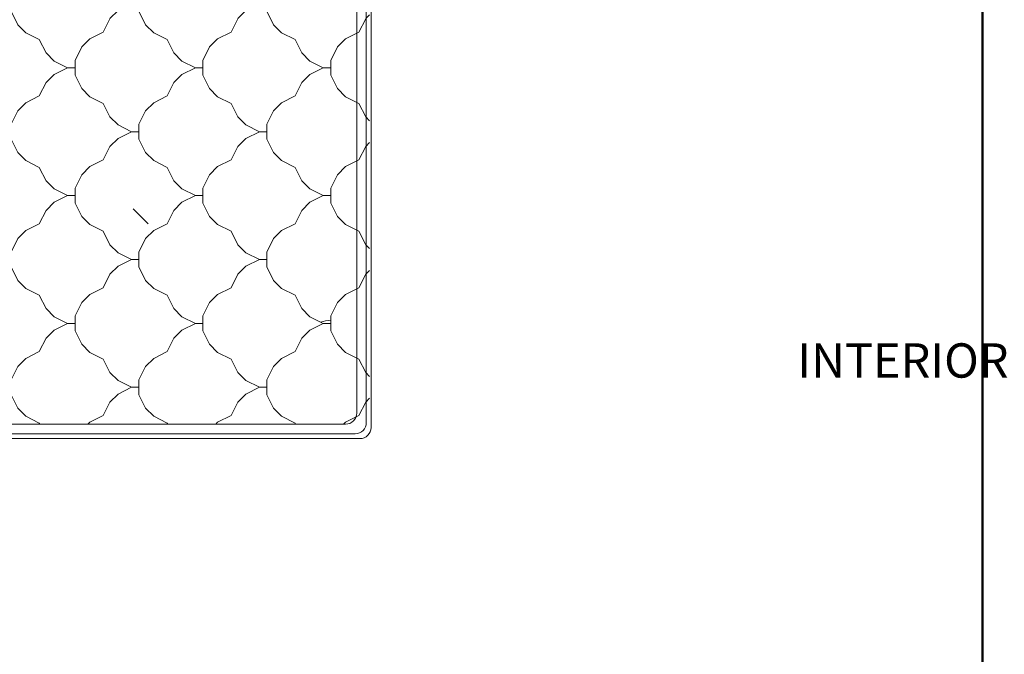
# Model space of a CAD drawing. Units: inches. Extents: x 513 to 1142, y 396 to 927.
# Tile 8 of 31: x 628 to 743, y 746 to 820. Entities that reach past the tile are written whole.
import ezdxf

# ---------------------------------------------------------------- set-up
doc = ezdxf.new("R2010")
doc.units = ezdxf.units.IN
doc.header["$MEASUREMENT"] = 0
doc.linetypes.add('DASHED', pattern=[0.75, 0.5, -0.25])
for name, color, linetype, lineweight in [('A-ANNO-DIMS', 2, 'DASHED', 18), ('A-WALL', 7, 'Continuous', 50), ('furniture', 92, 'Continuous', 18)]:
    doc.layers.add(name, color=color, linetype=linetype, lineweight=lineweight)
doc.styles.get("Standard").update_dxf_attribs({"font": 'arial.ttf'})
doc.dimstyles.get("Standard").update_dxf_attribs({"dimtxt": 4, "dimasz": 0.18, "dimexe": 0.18, "dimexo": 0.0625, "dimgap": 0.09, "dimtad": 0, "dimtih": 1, "dimtoh": 1, "dimdec": 0, "dimrnd": 6, "dimzin": 0, "dimdsep": 46, "dimlunit": 3, "dimtxsty": 'Standard', "dimcen": 0.09, "dimadec": 0, "dimazin": 0, "dimtfac": 1, "dimtdec": 0, "dimtofl": 0, "dimtmove": 0, "dimatfit": 3, "dimfxl": 1, "dimtolj": 1, "dimtzin": 0, "dimarcsym": 0})

# ---------------------------------------------------------------- blocks, each defined once
blk = doc.blocks.new('A$C029D5C69')
for p, q in [((0.4164, 2.0693), (0.4164, 2.0066)), ((2.2315, 2.0693), (0.4164, 2.0693)), ((2.2315, 2.0066), (2.2315, 2.0693)), ((0, 1.606), (0, 2.0066)), ((0, 2.0066), (0.505, 2.0066)), ((0.0151, 1.6211), (0.0151, 1.9915)), ((0.0151, 1.9915), (0.4899, 1.9915)), ((0.4164, 2.0066), (2.2315, 2.0066)), ((0.4899, 1.9915), (0.4899, 1.6211)), ((0.505, 2.0066), (0.505, 1.606)), ((0.5252, 0.0351), (0.5252, 2.0066)), ((0.5403, 0.0502), (0.5403, 2.0066)), ((0.5706, 0.0805), (0.5706, 2.0066)), ((0.6869, 1.966), (0.6666, 2.0066)), ((0.7072, 2.0066), (0.6869, 1.966)), ((1.0902, 1.966), (1.0699, 2.0066)), ((1.1106, 2.0066), (1.0902, 1.966)), ((2.1114, 2.0087), (2.1114, 0.0351)), ((2.6479, 2.0066), (2.1429, 2.0066)), ((2.1429, 2.0066), (2.1429, 1.606)), ((2.6328, 1.9915), (2.158, 1.9915)), ((2.158, 1.9915), (2.158, 1.6211)), ((2.6328, 1.6211), (2.6328, 1.9915)), ((2.6479, 1.606), (2.6479, 2.0066)), ((0.2689, 1.9609), (0.2689, 1.6764)), ((0.6869, 1.9425), (0.6869, 1.966)), ((0.6869, 1.9425), (0.6869, 1.966)), ((1.0902, 1.9425), (1.0902, 1.966)), ((1.0902, 1.9425), (1.0902, 1.966)), ((1.8954, 1.9865), (1.3081, 1.9865)), ((1.8954, 1.9713), (1.3339, 1.9713)), ((1.3849, 1.9713), (1.3656, 1.952)), ((1.3945, 1.9713), (1.3714, 1.9483)), ((1.4249, 1.945), (1.3986, 1.9713)), ((1.4288, 1.9507), (1.4081, 1.9713)), ((1.487, 1.9713), (1.4664, 1.9507)), ((1.4966, 1.9713), (1.4703, 1.945)), ((1.527, 1.945), (1.5007, 1.9713)), ((1.5309, 1.9507), (1.5102, 1.9713)), ((1.5891, 1.9713), (1.5685, 1.9507)), ((1.5987, 1.9713), (1.5724, 1.945)), ((1.6291, 1.945), (1.6028, 1.9713)), ((1.633, 1.9507), (1.6123, 1.9713)), ((1.6912, 1.9713), (1.6706, 1.9507)), ((1.7008, 1.9713), (1.6745, 1.945)), ((1.7312, 1.945), (1.7049, 1.9713)), ((1.7351, 1.9507), (1.7144, 1.9713)), ((1.7933, 1.9713), (1.7727, 1.9507)), ((1.8029, 1.9713), (1.7766, 1.945)), ((1.8333, 1.945), (1.807, 1.9713)), ((1.8372, 1.9507), (1.8165, 1.9713)), ((1.8954, 1.9713), (1.8748, 1.9507)), ((1.9043, 1.9707), (1.8787, 1.945)), ((1.9354, 1.945), (1.9114, 1.969)), ((2.379, 1.9609), (2.379, 1.6764)), ((0.6634, 1.9425), (0.621, 1.9213)), ((0.6634, 1.9425), (0.621, 1.9213)), ((0.6869, 1.9425), (0.6634, 1.9425)), ((0.6869, 1.9425), (0.7104, 1.9425)), ((0.7528, 1.9213), (0.7104, 1.9425)), ((0.7528, 1.9213), (0.7104, 1.9425)), ((1.0668, 1.9425), (1.0244, 1.9213)), ((1.0668, 1.9425), (1.0244, 1.9213)), ((1.0902, 1.9425), (1.0668, 1.9425)), ((1.0902, 1.9425), (1.1137, 1.9425)), ((1.1561, 1.9213), (1.1137, 1.9425)), ((1.1561, 1.9213), (1.1137, 1.9425)), ((1.4249, 1.945), (1.4059, 1.926)), ((1.4288, 1.9394), (1.4116, 1.9222)), ((1.4476, 1.9507), (1.4288, 1.9507)), ((1.4288, 1.9393), (1.4476, 1.9393)), ((1.4476, 1.9507), (1.4664, 1.9507)), ((1.4664, 1.9393), (1.4476, 1.9393)), ((1.493, 1.9128), (1.4664, 1.9394)), ((1.4986, 1.9167), (1.4703, 1.945)), ((1.527, 1.945), (1.4986, 1.9167)), ((1.5309, 1.9394), (1.5043, 1.9128)), ((1.5497, 1.9507), (1.5309, 1.9507)), ((1.5309, 1.9393), (1.5497, 1.9393)), ((1.5497, 1.9507), (1.5685, 1.9507)), ((1.5685, 1.9393), (1.5497, 1.9393)), ((1.595, 1.9128), (1.5685, 1.9394)), ((1.6007, 1.9167), (1.5724, 1.945)), ((1.6291, 1.945), (1.6007, 1.9167)), ((1.633, 1.9394), (1.6064, 1.9128)), ((1.6518, 1.9507), (1.633, 1.9507)), ((1.633, 1.9393), (1.6518, 1.9393)), ((1.6518, 1.9507), (1.6706, 1.9507)), ((1.6706, 1.9393), (1.6518, 1.9393)), ((1.6971, 1.9128), (1.6706, 1.9394)), ((1.7028, 1.9167), (1.6745, 1.945)), ((1.7312, 1.945), (1.7028, 1.9167)), ((1.7351, 1.9394), (1.7085, 1.9128)), ((1.7539, 1.9507), (1.7351, 1.9507)), ((1.7351, 1.9393), (1.7539, 1.9393)), ((1.7539, 1.9507), (1.7727, 1.9507)), ((1.7727, 1.9393), (1.7539, 1.9393)), ((1.7992, 1.9128), (1.7727, 1.9394)), ((1.8049, 1.9167), (1.7766, 1.945)), ((1.8333, 1.945), (1.8049, 1.9167)), ((1.8372, 1.9394), (1.8106, 1.9128)), ((1.856, 1.9507), (1.8372, 1.9507)), ((1.8372, 1.9393), (1.856, 1.9393)), ((1.856, 1.9507), (1.8748, 1.9507)), ((1.8748, 1.9393), (1.856, 1.9393)), ((1.9013, 1.9128), (1.8748, 1.9394)), ((1.907, 1.9167), (1.8787, 1.945)), ((1.9354, 1.945), (1.907, 1.9167)), ((1.9393, 1.9394), (1.9127, 1.9128)), ((1.9393, 1.9393), (1.9404, 1.9393)), ((1.9414, 1.688), (1.9414, 1.931)), ((1.9565, 1.688), (1.9565, 1.931)), ((0.5955, 1.8958), (0.5743, 1.8534)), ((0.621, 1.9213), (0.5955, 1.8958)), ((0.7783, 1.8958), (0.7528, 1.9213)), ((0.7995, 1.8534), (0.7783, 1.8958)), ((0.9989, 1.8958), (0.9777, 1.8534)), ((1.0243, 1.9213), (0.9988, 1.8958)), ((1.1816, 1.8958), (1.1561, 1.9213)), ((1.2028, 1.8534), (1.1816, 1.8958)), ((1.493, 1.8752), (1.493, 1.9128)), ((1.5043, 1.8752), (1.5043, 1.9128)), ((1.595, 1.8752), (1.595, 1.9128)), ((1.6064, 1.8752), (1.6064, 1.9128)), ((1.6971, 1.8752), (1.6971, 1.9128)), ((1.7085, 1.8752), (1.7085, 1.9128)), ((1.7992, 1.8752), (1.7992, 1.9128)), ((1.8106, 1.8752), (1.8106, 1.9128)), ((1.9013, 1.8752), (1.9013, 1.9128)), ((1.9127, 1.8752), (1.9127, 1.9128)), ((1.493, 1.8752), (1.4867, 1.869)), ((1.4986, 1.8713), (1.4922, 1.8648)), ((1.527, 1.8429), (1.4986, 1.8713)), ((1.5309, 1.8486), (1.5043, 1.8752)), ((1.595, 1.8752), (1.5685, 1.8486)), ((1.6007, 1.8713), (1.5724, 1.8429)), ((1.6291, 1.8429), (1.6007, 1.8713)), ((1.633, 1.8486), (1.6064, 1.8752)), ((1.6971, 1.8752), (1.6706, 1.8486)), ((1.7028, 1.8713), (1.6745, 1.8429)), ((1.7312, 1.8429), (1.7028, 1.8713)), ((1.7351, 1.8486), (1.7085, 1.8752)), ((1.7992, 1.8752), (1.7727, 1.8486)), ((1.8049, 1.8713), (1.7766, 1.8429)), ((1.8333, 1.8429), (1.8049, 1.8713)), ((1.8372, 1.8486), (1.8106, 1.8752)), ((1.9013, 1.8752), (1.8748, 1.8486)), ((1.907, 1.8713), (1.8787, 1.8429)), ((1.9354, 1.8429), (1.907, 1.8713)), ((1.9393, 1.8486), (1.9127, 1.8752)), ((0.5743, 1.8534), (0.5706, 1.8515)), ((0.5743, 1.8534), (0.5706, 1.8515)), ((0.8419, 1.8322), (0.7995, 1.8534)), ((0.8419, 1.8322), (0.7995, 1.8534)), ((0.9777, 1.8534), (0.9353, 1.8322)), ((0.9777, 1.8534), (0.9353, 1.8322)), ((1.2452, 1.8322), (1.2028, 1.8534)), ((1.2452, 1.8322), (1.2028, 1.8534)), ((1.527, 1.8429), (1.5242, 1.8401)), ((1.5309, 1.8373), (1.5295, 1.8359)), ((1.5497, 1.8486), (1.5309, 1.8486)), ((1.5309, 1.8373), (1.5497, 1.8373)), ((1.5497, 1.8486), (1.5685, 1.8486)), ((1.5685, 1.8373), (1.5497, 1.8373)), ((1.595, 1.8107), (1.5685, 1.8373)), ((1.6007, 1.8146), (1.5724, 1.8429)), ((1.6291, 1.8429), (1.6007, 1.8146)), ((1.633, 1.8373), (1.6064, 1.8107)), ((1.6518, 1.8486), (1.633, 1.8486)), ((1.633, 1.8373), (1.6518, 1.8373)), ((1.6518, 1.8486), (1.6706, 1.8486)), ((1.6706, 1.8373), (1.6518, 1.8373)), ((1.6971, 1.8107), (1.6706, 1.8373)), ((1.7028, 1.8146), (1.6745, 1.8429)), ((1.7312, 1.8429), (1.7028, 1.8146)), ((1.7351, 1.8373), (1.7085, 1.8107)), ((1.7539, 1.8486), (1.7351, 1.8486)), ((1.7351, 1.8373), (1.7539, 1.8373)), ((1.7539, 1.8486), (1.7727, 1.8486)), ((1.7727, 1.8373), (1.7539, 1.8373)), ((1.7992, 1.8107), (1.7727, 1.8373)), ((1.8049, 1.8146), (1.7766, 1.8429)), ((1.8333, 1.8429), (1.8049, 1.8146)), ((1.8372, 1.8373), (1.8106, 1.8107)), ((1.856, 1.8486), (1.8372, 1.8486)), ((1.8372, 1.8373), (1.856, 1.8373)), ((1.856, 1.8486), (1.8748, 1.8486)), ((1.8748, 1.8373), (1.856, 1.8373)), ((1.9013, 1.8107), (1.8748, 1.8373)), ((1.907, 1.8146), (1.8787, 1.8429)), ((1.9354, 1.8429), (1.907, 1.8146)), ((1.9393, 1.8373), (1.9127, 1.8107)), ((1.9414, 1.8486), (1.9393, 1.8486)), ((1.9393, 1.8373), (1.9414, 1.8373)), ((0.1267, 1.8186), (0.4111, 1.8186)), ((0.8674, 1.8067), (0.8419, 1.8322)), ((0.8886, 1.7643), (0.8674, 1.8067)), ((0.9098, 1.8067), (0.8886, 1.7643)), ((0.9352, 1.8322), (0.9097, 1.8067)), ((1.2707, 1.8067), (1.2452, 1.8322)), ((1.2919, 1.7643), (1.2707, 1.8067)), ((1.595, 1.7806), (1.595, 1.8107)), ((1.6064, 1.7731), (1.6064, 1.8107)), ((1.6971, 1.7731), (1.6971, 1.8107)), ((1.7085, 1.7731), (1.7085, 1.8107)), ((1.7992, 1.7731), (1.7992, 1.8107)), ((1.8106, 1.7731), (1.8106, 1.8107)), ((1.9013, 1.7731), (1.9013, 1.8107)), ((1.9127, 1.7731), (1.9127, 1.8107)), ((2.2367, 1.8186), (2.5212, 1.8186)), ((1.2981, 1.7768), (1.2919, 1.7643)), ((1.633, 1.7465), (1.6064, 1.7731)), ((1.6971, 1.7731), (1.6706, 1.7465)), ((1.7351, 1.7465), (1.7085, 1.7731)), ((1.7992, 1.7731), (1.7727, 1.7465)), ((1.8372, 1.7465), (1.8106, 1.7731)), ((1.9013, 1.7731), (1.8748, 1.7465)), ((1.9393, 1.7465), (1.9127, 1.7731)), ((0.8651, 1.7408), (0.8227, 1.7196)), ((0.8651, 1.7408), (0.8227, 1.7196)), ((0.912, 1.7408), (0.8651, 1.7408)), ((0.8886, 1.7408), (0.8886, 1.7643)), ((0.9544, 1.7196), (0.912, 1.7408)), ((0.9544, 1.7196), (0.912, 1.7408)), ((1.2684, 1.7408), (1.226, 1.7196)), ((1.2684, 1.7408), (1.226, 1.7196)), ((1.2885, 1.7408), (1.2684, 1.7408)), ((1.2919, 1.7519), (1.2919, 1.7643)), ((1.6518, 1.7465), (1.633, 1.7465)), ((1.6518, 1.7465), (1.6706, 1.7465)), ((1.7028, 1.7692), (1.6745, 1.7408)), ((1.7028, 1.7125), (1.6745, 1.7408)), ((1.7312, 1.7408), (1.7028, 1.7692)), ((1.7312, 1.7408), (1.7028, 1.7125)), ((1.7539, 1.7465), (1.7351, 1.7465)), ((1.7539, 1.7465), (1.7727, 1.7465)), ((1.8049, 1.7692), (1.7766, 1.7408)), ((1.8049, 1.7125), (1.7766, 1.7408)), ((1.8333, 1.7408), (1.8049, 1.7692)), ((1.8333, 1.7408), (1.8049, 1.7125)), ((1.856, 1.7465), (1.8372, 1.7465)), ((1.856, 1.7465), (1.8748, 1.7465)), ((1.907, 1.7692), (1.8787, 1.7408)), ((1.907, 1.7125), (1.8787, 1.7408)), ((1.9354, 1.7408), (1.907, 1.7692)), ((1.9354, 1.7408), (1.907, 1.7125)), ((1.9414, 1.7465), (1.9393, 1.7465)), ((0.8227, 1.7196), (0.7972, 1.6941)), ((0.98, 1.6941), (0.9545, 1.7196)), ((1.226, 1.7196), (1.2005, 1.6941)), ((1.6443, 1.7352), (1.6518, 1.7352)), ((1.6706, 1.7352), (1.6518, 1.7352)), ((1.6971, 1.7086), (1.6706, 1.7352)), ((1.6971, 1.682), (1.6971, 1.7086)), ((1.7351, 1.7352), (1.7085, 1.7086)), ((1.7085, 1.671), (1.7085, 1.7086)), ((1.7351, 1.7352), (1.7539, 1.7352)), ((1.7727, 1.7352), (1.7539, 1.7352)), ((1.7992, 1.7086), (1.7727, 1.7352)), ((1.7992, 1.671), (1.7992, 1.7086)), ((1.8372, 1.7352), (1.8106, 1.7086)), ((1.8106, 1.671), (1.8106, 1.7086)), ((1.8372, 1.7352), (1.856, 1.7352)), ((1.8748, 1.7352), (1.856, 1.7352)), ((1.9013, 1.7086), (1.8748, 1.7352)), ((1.9013, 1.671), (1.9013, 1.7086)), ((1.9393, 1.7352), (1.9127, 1.7086)), ((1.9127, 1.671), (1.9127, 1.7086)), ((1.9393, 1.7352), (1.9414, 1.7352)), ((0.5766, 1.6941), (0.5706, 1.7002)), ((0.5978, 1.6517), (0.5766, 1.6941)), ((0.7972, 1.6941), (0.776, 1.6517)), ((1.0011, 1.6517), (0.9799, 1.6941)), ((1.2005, 1.6941), (1.1793, 1.6517)), ((2.5551, 1.6275), (2.5551, 1.696)), ((0.6402, 1.6305), (0.5978, 1.6517)), ((0.6402, 1.6305), (0.5978, 1.6517)), ((0.776, 1.6517), (0.7336, 1.6305)), ((0.776, 1.6517), (0.7336, 1.6305)), ((1.0435, 1.6305), (1.0011, 1.6517)), ((1.0435, 1.6305), (1.0011, 1.6517)), ((1.1793, 1.6517), (1.1369, 1.6305)), ((1.1793, 1.6517), (1.1369, 1.6305)), ((1.7318, 1.6477), (1.7085, 1.671)), ((1.8961, 1.6477), (1.7289, 1.6477)), ((1.7992, 1.671), (1.7759, 1.6477)), ((1.8049, 1.6671), (1.7855, 1.6477)), ((1.8244, 1.6477), (1.8049, 1.6671)), ((1.8339, 1.6477), (1.8106, 1.671)), ((1.9013, 1.671), (1.878, 1.6477)), ((1.907, 1.6671), (1.8876, 1.6477)), ((1.9202, 1.6539), (1.907, 1.6671)), ((1.926, 1.6577), (1.9127, 1.671)), ((0.4899, 1.6211), (0.0151, 1.6211)), ((0.6657, 1.605), (0.6402, 1.6305)), ((0.7336, 1.6305), (0.7081, 1.605)), ((1.0691, 1.605), (1.0436, 1.6305)), ((1.1369, 1.6305), (1.1114, 1.605)), ((1.8961, 1.6325), (1.7422, 1.6325)), ((2.158, 1.6211), (2.6328, 1.6211)), ((0.505, 1.606), (0, 1.606)), ((0.6869, 1.5626), (0.6657, 1.605)), ((0.7081, 1.605), (0.6869, 1.5626)), ((1.0902, 1.5626), (1.069, 1.605)), ((1.1114, 1.605), (1.0902, 1.5626)), ((2.1429, 1.606), (2.6479, 1.606)), ((0.6869, 1.5392), (0.6869, 1.5626)), ((0.6869, 1.5392), (0.6869, 1.5626)), ((1.0902, 1.5392), (1.0902, 1.5626)), ((1.0902, 1.5392), (1.0902, 1.5626)), ((0.6634, 1.5391), (0.621, 1.5179)), ((0.6634, 1.5391), (0.621, 1.5179)), ((0.6869, 1.5392), (0.6634, 1.5392)), ((0.6869, 1.5392), (0.7104, 1.5392)), ((0.7528, 1.5179), (0.7104, 1.5391)), ((0.7528, 1.5179), (0.7104, 1.5391)), ((1.0668, 1.5391), (1.0244, 1.5179)), ((1.0668, 1.5391), (1.0244, 1.5179)), ((1.0902, 1.5392), (1.0668, 1.5392)), ((1.0902, 1.5392), (1.1137, 1.5392)), ((1.1561, 1.5179), (1.1137, 1.5391)), ((1.1561, 1.5179), (1.1137, 1.5391)), ((1.4534, 1.5308), (1.4277, 1.5179)), ((1.4534, 1.5308), (1.4277, 1.5179)), ((0.5955, 1.4925), (0.5743, 1.4501)), ((0.621, 1.5179), (0.5955, 1.4924)), ((0.7783, 1.4924), (0.7528, 1.5179)), ((0.7995, 1.4501), (0.7783, 1.4925)), ((0.9989, 1.4925), (0.9777, 1.4501)), ((1.0243, 1.5179), (0.9988, 1.4924)), ((1.1816, 1.4924), (1.1561, 1.5179)), ((1.2028, 1.4501), (1.1816, 1.4925)), ((1.4022, 1.4925), (1.381, 1.4501)), ((1.4277, 1.5179), (1.4022, 1.4924)), ((1.6062, 1.4501), (1.5966, 1.4692)), ((0.5743, 1.45), (0.5706, 1.4481)), ((0.5743, 1.45), (0.5706, 1.4481)), ((0.8419, 1.4288), (0.7995, 1.45)), ((0.8419, 1.4288), (0.7995, 1.45)), ((0.8674, 1.4033), (0.8419, 1.4288)), ((0.9352, 1.4288), (0.9097, 1.4033)), ((0.9777, 1.45), (0.9353, 1.4288)), ((0.9777, 1.45), (0.9353, 1.4288)), ((1.2452, 1.4288), (1.2028, 1.45)), ((1.2452, 1.4288), (1.2028, 1.45)), ((1.2707, 1.4033), (1.2452, 1.4288)), ((1.3386, 1.4288), (1.3131, 1.4033)), ((1.381, 1.45), (1.3386, 1.4288)), ((1.381, 1.45), (1.3386, 1.4288)), ((1.6486, 1.4288), (1.6062, 1.45)), ((1.6486, 1.4288), (1.6062, 1.45)), ((1.6741, 1.4033), (1.6486, 1.4288)), ((0.5403, 1.4117), (0.5706, 1.4117)), ((0.8886, 1.361), (0.8674, 1.4034)), ((0.9098, 1.4034), (0.8886, 1.361)), ((1.2919, 1.361), (1.2707, 1.4034)), ((1.3131, 1.4034), (1.2919, 1.361)), ((1.6953, 1.361), (1.6741, 1.4034)), ((1.714, 1.3984), (1.6953, 1.361)), ((0.8651, 1.3374), (0.8227, 1.3162)), ((0.8651, 1.3374), (0.8227, 1.3162)), ((0.912, 1.3375), (0.8651, 1.3375)), ((0.8886, 1.3375), (0.8886, 1.3609)), ((0.9544, 1.3162), (0.912, 1.3374)), ((0.9544, 1.3162), (0.912, 1.3374)), ((1.2684, 1.3374), (1.226, 1.3162)), ((1.2684, 1.3374), (1.226, 1.3162)), ((1.3154, 1.3375), (1.2684, 1.3375)), ((1.2919, 1.3375), (1.2919, 1.3609)), ((1.3578, 1.3162), (1.3154, 1.3374)), ((1.3578, 1.3162), (1.3154, 1.3374)), ((1.6718, 1.3374), (1.6294, 1.3162)), ((1.6718, 1.3374), (1.6294, 1.3162)), ((1.7187, 1.3375), (1.6718, 1.3375)), ((1.6953, 1.3375), (1.6953, 1.3609)), ((1.7611, 1.3162), (1.7187, 1.3374)), ((1.7611, 1.3162), (1.7187, 1.3374)), ((0.8227, 1.3163), (0.7972, 1.2908)), ((0.98, 1.2908), (0.9545, 1.3163)), ((1.226, 1.3163), (1.2005, 1.2908)), ((1.3833, 1.2908), (1.3578, 1.3163)), ((1.6294, 1.3163), (1.6039, 1.2908)), ((1.7867, 1.2908), (1.7611, 1.3163)), ((0.5766, 1.2908), (0.5706, 1.2968)), ((0.5978, 1.2484), (0.5766, 1.2908)), ((0.7972, 1.2908), (0.776, 1.2484)), ((1.0011, 1.2484), (0.9799, 1.2908)), ((1.2005, 1.2908), (1.1793, 1.2484)), ((1.4045, 1.2484), (1.3833, 1.2908)), ((1.6039, 1.2908), (1.5827, 1.2484)), ((1.8078, 1.2484), (1.7866, 1.2908)), ((0.6402, 1.2271), (0.5978, 1.2483)), ((0.6402, 1.2271), (0.5978, 1.2483)), ((0.776, 1.2483), (0.7336, 1.2271)), ((0.776, 1.2483), (0.7336, 1.2271)), ((1.0435, 1.2271), (1.0011, 1.2483)), ((1.0435, 1.2271), (1.0011, 1.2483)), ((1.1793, 1.2483), (1.1369, 1.2271)), ((1.1793, 1.2483), (1.1369, 1.2271)), ((1.4469, 1.2271), (1.4045, 1.2483)), ((1.4469, 1.2271), (1.4045, 1.2483)), ((1.5827, 1.2483), (1.5403, 1.2271)), ((1.5827, 1.2483), (1.5403, 1.2271)), ((1.8502, 1.2271), (1.8078, 1.2483)), ((1.8502, 1.2271), (1.8078, 1.2483)), ((0.6657, 1.2017), (0.6402, 1.2272)), ((0.7336, 1.2272), (0.7081, 1.2017)), ((1.0691, 1.2017), (1.0436, 1.2272)), ((1.1369, 1.2272), (1.1114, 1.2017)), ((1.4724, 1.2017), (1.4469, 1.2272)), ((1.5403, 1.2272), (1.5148, 1.2017)), ((1.8758, 1.2017), (1.8503, 1.2272)), ((0.5403, 1.21), (0.5706, 1.21)), ((0.6869, 1.1593), (0.6657, 1.2017)), ((0.7081, 1.2017), (0.6869, 1.1593)), ((1.0902, 1.1593), (1.069, 1.2017)), ((1.1114, 1.2017), (1.0902, 1.1593)), ((1.4936, 1.1593), (1.4724, 1.2017)), ((1.5148, 1.2017), (1.4936, 1.1593)), ((1.8969, 1.1593), (1.8757, 1.2017)), ((1.9181, 1.2017), (1.8969, 1.1593)), ((1.9215, 1.2051), (1.9181, 1.2017)), ((0.6869, 1.1358), (0.6869, 1.1593)), ((0.6869, 1.1358), (0.6869, 1.1593)), ((1.0902, 1.1358), (1.0902, 1.1593)), ((1.0902, 1.1358), (1.0902, 1.1593)), ((1.4936, 1.1358), (1.4936, 1.1593)), ((1.4936, 1.1358), (1.4936, 1.1593)), ((1.8969, 1.1358), (1.8969, 1.1593)), ((1.8969, 1.1358), (1.8969, 1.1593)), ((0.6634, 1.1358), (0.621, 1.1146)), ((0.6634, 1.1358), (0.621, 1.1146)), ((0.6869, 1.1358), (0.6634, 1.1358)), ((0.6869, 1.1358), (0.7104, 1.1358)), ((0.7528, 1.1146), (0.7104, 1.1358)), ((0.7528, 1.1146), (0.7104, 1.1358)), ((1.0668, 1.1358), (1.0244, 1.1146)), ((1.0668, 1.1358), (1.0244, 1.1146)), ((1.0902, 1.1358), (1.0668, 1.1358)), ((1.0902, 1.1358), (1.1137, 1.1358)), ((1.1561, 1.1146), (1.1137, 1.1358)), ((1.1561, 1.1146), (1.1137, 1.1358)), ((1.4701, 1.1358), (1.4277, 1.1146)), ((1.4701, 1.1358), (1.4277, 1.1146)), ((1.4936, 1.1358), (1.4701, 1.1358)), ((1.4936, 1.1358), (1.5171, 1.1358)), ((1.5595, 1.1146), (1.5171, 1.1358)), ((1.5595, 1.1146), (1.5171, 1.1358)), ((1.8735, 1.1358), (1.8311, 1.1146)), ((1.8735, 1.1358), (1.8311, 1.1146)), ((1.8969, 1.1358), (1.8735, 1.1358)), ((1.8969, 1.1358), (1.9204, 1.1358)), ((1.9628, 1.1146), (1.9204, 1.1358)), ((1.9628, 1.1146), (1.9204, 1.1358)), ((0.5955, 1.0891), (0.5743, 1.0467)), ((0.621, 1.1146), (0.5955, 1.0891)), ((0.7783, 1.0891), (0.7528, 1.1146)), ((0.7995, 1.0467), (0.7783, 1.0891)), ((0.9989, 1.0891), (0.9777, 1.0467)), ((1.0243, 1.1146), (0.9988, 1.0891)), ((1.1816, 1.0891), (1.1561, 1.1146)), ((1.2028, 1.0467), (1.1816, 1.0891)), ((1.4022, 1.0891), (1.381, 1.0467)), ((1.4277, 1.1146), (1.4022, 1.0891)), ((1.585, 1.0891), (1.5595, 1.1146)), ((1.6062, 1.0467), (1.585, 1.0891)), ((1.8056, 1.0891), (1.7844, 1.0467)), ((1.831, 1.1146), (1.8055, 1.0891)), ((1.9883, 1.0891), (1.9628, 1.1146)), ((2.0095, 1.0467), (1.9883, 1.0891)), ((0.5743, 1.0467), (0.5706, 1.0448)), ((0.5743, 1.0467), (0.5706, 1.0448)), ((0.8419, 1.0255), (0.7995, 1.0467)), ((0.8419, 1.0255), (0.7995, 1.0467)), ((0.8674, 1), (0.8419, 1.0255)), ((0.9352, 1.0255), (0.9097, 1)), ((0.9777, 1.0467), (0.9353, 1.0255)), ((0.9777, 1.0467), (0.9353, 1.0255)), ((1.2452, 1.0255), (1.2028, 1.0467)), ((1.2452, 1.0255), (1.2028, 1.0467)), ((1.2707, 1), (1.2452, 1.0255)), ((1.3386, 1.0255), (1.3131, 1)), ((1.381, 1.0467), (1.3386, 1.0255)), ((1.381, 1.0467), (1.3386, 1.0255)), ((1.6486, 1.0255), (1.6062, 1.0467)), ((1.6486, 1.0255), (1.6062, 1.0467)), ((1.6741, 1), (1.6486, 1.0255)), ((1.7419, 1.0255), (1.7164, 1)), ((1.7844, 1.0467), (1.742, 1.0255)), ((1.7844, 1.0467), (1.742, 1.0255)), ((2.0276, 1.0376), (2.0095, 1.0467)), ((2.0276, 1.0376), (2.0095, 1.0467)), ((0.8886, 0.9576), (0.8674, 1)), ((0.9098, 1), (0.8886, 0.9576)), ((1.2919, 0.9576), (1.2707, 1)), ((1.3131, 1), (1.2919, 0.9576)), ((1.6953, 0.9576), (1.6741, 1)), ((1.7165, 1), (1.6953, 0.9576)), ((0.8651, 0.9341), (0.8227, 0.9129)), ((0.8651, 0.9341), (0.8227, 0.9129)), ((0.912, 0.9341), (0.8651, 0.9341)), ((0.8886, 0.9341), (0.8886, 0.9576)), ((0.9544, 0.9129), (0.912, 0.9341)), ((0.9544, 0.9129), (0.912, 0.9341)), ((1.2684, 0.9341), (1.226, 0.9129)), ((1.2684, 0.9341), (1.226, 0.9129)), ((1.3154, 0.9341), (1.2684, 0.9341)), ((1.2919, 0.9341), (1.2919, 0.9576)), ((1.3578, 0.9129), (1.3154, 0.9341)), ((1.3578, 0.9129), (1.3154, 0.9341)), ((1.6718, 0.9341), (1.6294, 0.9129)), ((1.6718, 0.9341), (1.6294, 0.9129)), ((1.7187, 0.9341), (1.6718, 0.9341)), ((1.6953, 0.9341), (1.6953, 0.9576)), ((1.7611, 0.9129), (1.7187, 0.9341)), ((1.7611, 0.9129), (1.7187, 0.9341)), ((2.066, 0.9457), (2.066, 0.0805)), ((0.8227, 0.9129), (0.7972, 0.8874)), ((0.98, 0.8874), (0.9545, 0.9129)), ((1.226, 0.9129), (1.2005, 0.8874)), ((1.3833, 0.8874), (1.3578, 0.9129)), ((1.6294, 0.9129), (1.6039, 0.8874)), ((1.7867, 0.8874), (1.7611, 0.9129)), ((2.0327, 0.9129), (2.0072, 0.8874)), ((2.066, 0.9295), (2.0327, 0.9129)), ((2.066, 0.9295), (2.0327, 0.9129)), ((0.5766, 0.8874), (0.5706, 0.8935)), ((0.5978, 0.845), (0.5766, 0.8874)), ((0.7972, 0.8874), (0.776, 0.845)), ((1.0011, 0.845), (0.9799, 0.8874)), ((1.2005, 0.8874), (1.1793, 0.845)), ((1.4045, 0.845), (1.3833, 0.8874)), ((1.6039, 0.8874), (1.5827, 0.845)), ((1.8078, 0.845), (1.7866, 0.8874)), ((2.0072, 0.8874), (1.986, 0.845)), ((0.6402, 0.8238), (0.5978, 0.845)), ((0.6402, 0.8238), (0.5978, 0.845)), ((0.776, 0.845), (0.7336, 0.8238)), ((0.776, 0.845), (0.7336, 0.8238)), ((1.0435, 0.8238), (1.0011, 0.845)), ((1.0435, 0.8238), (1.0011, 0.845)), ((1.1793, 0.845), (1.1369, 0.8238)), ((1.1793, 0.845), (1.1369, 0.8238)), ((1.4469, 0.8238), (1.4045, 0.845)), ((1.4469, 0.8238), (1.4045, 0.845)), ((1.5827, 0.845), (1.5403, 0.8238)), ((1.5827, 0.845), (1.5403, 0.8238)), ((1.8502, 0.8238), (1.8078, 0.845)), ((1.8502, 0.8238), (1.8078, 0.845)), ((1.986, 0.845), (1.9436, 0.8238)), ((1.986, 0.845), (1.9436, 0.8238)), ((0.6657, 0.7983), (0.6402, 0.8238)), ((0.7336, 0.8238), (0.7081, 0.7983)), ((1.0691, 0.7983), (1.0436, 0.8238)), ((1.1369, 0.8238), (1.1114, 0.7983)), ((1.4724, 0.7983), (1.4469, 0.8238)), ((1.5403, 0.8238), (1.5148, 0.7983)), ((1.8758, 0.7983), (1.8503, 0.8238)), ((1.9436, 0.8238), (1.9181, 0.7983)), ((2.0962, 0.8369), (2.0962, 0.0502)), ((0.6869, 0.7559), (0.6657, 0.7983)), ((0.7081, 0.7983), (0.6869, 0.7559)), ((1.0902, 0.7559), (1.069, 0.7983)), ((1.1114, 0.7983), (1.0902, 0.7559)), ((1.4936, 0.7559), (1.4724, 0.7983)), ((1.5148, 0.7983), (1.4936, 0.7559)), ((1.8969, 0.7559), (1.8757, 0.7983)), ((1.9181, 0.7983), (1.8969, 0.7559)), ((0.6869, 0.7325), (0.6869, 0.7559)), ((0.6869, 0.7325), (0.6869, 0.7559)), ((1.0902, 0.7325), (1.0902, 0.7559)), ((1.0902, 0.7325), (1.0902, 0.7559)), ((1.2024, 0.7028), (1.2503, 0.7507)), ((1.4936, 0.7325), (1.4936, 0.7559)), ((1.4936, 0.7325), (1.4936, 0.7559)), ((1.8969, 0.7325), (1.8969, 0.7559)), ((1.8969, 0.7325), (1.8969, 0.7559)), ((0.6634, 0.7324), (0.621, 0.7112)), ((0.6634, 0.7324), (0.621, 0.7112)), ((0.6869, 0.7325), (0.6634, 0.7325)), ((0.6869, 0.7325), (0.7104, 0.7325)), ((0.7528, 0.7112), (0.7104, 0.7324)), ((0.7528, 0.7112), (0.7104, 0.7324)), ((1.0668, 0.7324), (1.0244, 0.7112)), ((1.0668, 0.7324), (1.0244, 0.7112)), ((1.0902, 0.7325), (1.0668, 0.7325)), ((1.0902, 0.7325), (1.1137, 0.7325)), ((1.1561, 0.7112), (1.1137, 0.7324)), ((1.1561, 0.7112), (1.1137, 0.7324)), ((1.4701, 0.7324), (1.4277, 0.7112)), ((1.4701, 0.7324), (1.4277, 0.7112)), ((1.4936, 0.7325), (1.4701, 0.7325)), ((1.4936, 0.7325), (1.5171, 0.7325)), ((1.5595, 0.7112), (1.5171, 0.7324)), ((1.5595, 0.7112), (1.5171, 0.7324)), ((1.8735, 0.7324), (1.8311, 0.7112)), ((1.8735, 0.7324), (1.8311, 0.7112)), ((1.8969, 0.7325), (1.8735, 0.7325)), ((1.8969, 0.7325), (1.9204, 0.7325)), ((1.9628, 0.7112), (1.9204, 0.7324)), ((1.9628, 0.7112), (1.9204, 0.7324)), ((0.5955, 0.6858), (0.5743, 0.6434)), ((0.621, 0.7113), (0.5955, 0.6858)), ((0.7783, 0.6858), (0.7528, 0.7113)), ((0.7995, 0.6434), (0.7783, 0.6858)), ((0.9989, 0.6858), (0.9777, 0.6434)), ((1.0243, 0.7113), (0.9988, 0.6858)), ((1.1816, 0.6858), (1.1561, 0.7113)), ((1.2028, 0.6434), (1.1816, 0.6858)), ((1.4022, 0.6858), (1.381, 0.6434)), ((1.4277, 0.7113), (1.4022, 0.6858)), ((1.585, 0.6858), (1.5595, 0.7113)), ((1.6062, 0.6434), (1.585, 0.6858)), ((1.8056, 0.6858), (1.7844, 0.6434)), ((1.831, 0.7113), (1.8055, 0.6858)), ((1.9883, 0.6858), (1.9628, 0.7113)), ((2.0095, 0.6434), (1.9883, 0.6858)), ((0.5743, 0.6433), (0.5706, 0.6414)), ((0.5743, 0.6433), (0.5706, 0.6414)), ((0.8419, 0.6221), (0.7995, 0.6433)), ((0.8419, 0.6221), (0.7995, 0.6433)), ((0.8674, 0.5967), (0.8419, 0.6222)), ((0.9352, 0.6222), (0.9097, 0.5967)), ((0.9777, 0.6433), (0.9353, 0.6221)), ((0.9777, 0.6433), (0.9353, 0.6221)), ((1.2452, 0.6221), (1.2028, 0.6433)), ((1.2452, 0.6221), (1.2028, 0.6433)), ((1.2707, 0.5967), (1.2452, 0.6222)), ((1.3386, 0.6222), (1.3131, 0.5967)), ((1.381, 0.6433), (1.3386, 0.6221)), ((1.381, 0.6433), (1.3386, 0.6221)), ((1.6486, 0.6221), (1.6062, 0.6433)), ((1.6486, 0.6221), (1.6062, 0.6433)), ((1.6741, 0.5967), (1.6486, 0.6222)), ((1.7419, 0.6222), (1.7164, 0.5967)), ((1.7844, 0.6433), (1.742, 0.6221)), ((1.7844, 0.6433), (1.742, 0.6221)), ((2.0519, 0.6221), (2.0095, 0.6433)), ((2.0519, 0.6221), (2.0095, 0.6433)), ((2.066, 0.6081), (2.0519, 0.6222)), ((0.8886, 0.5543), (0.8674, 0.5967)), ((0.9098, 0.5967), (0.8886, 0.5543)), ((1.2919, 0.5543), (1.2707, 0.5967)), ((1.3131, 0.5967), (1.2919, 0.5543)), ((1.6953, 0.5543), (1.6741, 0.5967)), ((1.7165, 0.5967), (1.6953, 0.5543)), ((0.8651, 0.5308), (0.8227, 0.5096)), ((0.8651, 0.5308), (0.8227, 0.5096)), ((0.912, 0.5308), (0.8651, 0.5308)), ((0.8886, 0.5308), (0.8886, 0.5543)), ((0.9544, 0.5096), (0.912, 0.5308)), ((0.9544, 0.5096), (0.912, 0.5308)), ((1.2684, 0.5308), (1.226, 0.5096)), ((1.2684, 0.5308), (1.226, 0.5096)), ((1.3154, 0.5308), (1.2684, 0.5308)), ((1.2919, 0.5308), (1.2919, 0.5543)), ((1.3578, 0.5096), (1.3154, 0.5308)), ((1.3578, 0.5096), (1.3154, 0.5308)), ((1.6718, 0.5308), (1.6294, 0.5096)), ((1.6718, 0.5308), (1.6294, 0.5096)), ((1.7187, 0.5308), (1.6718, 0.5308)), ((1.6953, 0.5308), (1.6953, 0.5543)), ((1.7611, 0.5096), (1.7187, 0.5308)), ((1.7611, 0.5096), (1.7187, 0.5308)), ((0.8227, 0.5096), (0.7972, 0.4841)), ((0.98, 0.4841), (0.9545, 0.5096)), ((1.226, 0.5096), (1.2005, 0.4841)), ((1.3833, 0.4841), (1.3578, 0.5096)), ((1.6294, 0.5096), (1.6039, 0.4841)), ((1.7867, 0.4841), (1.7611, 0.5096)), ((2.0327, 0.5096), (2.0072, 0.4841)), ((2.066, 0.5262), (2.0327, 0.5096)), ((2.066, 0.5262), (2.0327, 0.5096)), ((0.5766, 0.4841), (0.5706, 0.4901)), ((0.5978, 0.4417), (0.5766, 0.4841)), ((0.7972, 0.4841), (0.776, 0.4417)), ((1.0011, 0.4417), (0.9799, 0.4841)), ((1.2005, 0.4841), (1.1793, 0.4417)), ((1.4045, 0.4417), (1.3833, 0.4841)), ((1.6039, 0.4841), (1.5827, 0.4417)), ((1.8078, 0.4417), (1.7866, 0.4841)), ((2.0072, 0.4841), (1.986, 0.4417)), ((0.6402, 0.4205), (0.5978, 0.4417)), ((0.6402, 0.4205), (0.5978, 0.4417)), ((0.776, 0.4417), (0.7336, 0.4205)), ((0.776, 0.4417), (0.7336, 0.4205)), ((1.0435, 0.4205), (1.0011, 0.4417)), ((1.0435, 0.4205), (1.0011, 0.4417)), ((1.1793, 0.4417), (1.1369, 0.4205)), ((1.1793, 0.4417), (1.1369, 0.4205)), ((1.4469, 0.4205), (1.4045, 0.4417)), ((1.4469, 0.4205), (1.4045, 0.4417)), ((1.5827, 0.4417), (1.5403, 0.4205)), ((1.5827, 0.4417), (1.5403, 0.4205)), ((1.8502, 0.4205), (1.8078, 0.4417)), ((1.8502, 0.4205), (1.8078, 0.4417)), ((1.986, 0.4417), (1.9436, 0.4205)), ((1.986, 0.4417), (1.9436, 0.4205)), ((0.6657, 0.395), (0.6402, 0.4205)), ((0.7336, 0.4205), (0.7081, 0.395)), ((1.0691, 0.395), (1.0436, 0.4205)), ((1.1369, 0.4205), (1.1114, 0.395)), ((1.4724, 0.395), (1.4469, 0.4205)), ((1.5403, 0.4205), (1.5148, 0.395)), ((1.8758, 0.395), (1.8503, 0.4205)), ((1.9436, 0.4205), (1.9181, 0.395)), ((0.6869, 0.3526), (0.6657, 0.395)), ((0.7081, 0.395), (0.6869, 0.3526)), ((1.0902, 0.3526), (1.069, 0.395)), ((1.1114, 0.395), (1.0902, 0.3526)), ((1.4936, 0.3526), (1.4724, 0.395)), ((1.5148, 0.395), (1.4936, 0.3526)), ((1.8969, 0.3526), (1.8757, 0.395)), ((1.9181, 0.395), (1.8969, 0.3526)), ((0.6869, 0.3291), (0.6869, 0.3526)), ((0.6869, 0.3291), (0.6869, 0.3526)), ((1.0902, 0.3291), (1.0902, 0.3526)), ((1.0902, 0.3291), (1.0902, 0.3526)), ((1.4936, 0.3291), (1.4936, 0.3526)), ((1.4936, 0.3291), (1.4936, 0.3526)), ((1.8969, 0.3291), (1.8969, 0.3526)), ((1.8969, 0.3291), (1.8969, 0.3526)), ((0.6634, 0.3291), (0.621, 0.3079)), ((0.6634, 0.3291), (0.621, 0.3079)), ((0.6869, 0.3291), (0.6634, 0.3291)), ((0.6869, 0.3291), (0.7104, 0.3291)), ((0.7528, 0.3079), (0.7104, 0.3291)), ((0.7528, 0.3079), (0.7104, 0.3291)), ((1.0668, 0.3291), (1.0244, 0.3079)), ((1.0668, 0.3291), (1.0244, 0.3079)), ((1.0902, 0.3291), (1.0668, 0.3291)), ((1.0902, 0.3291), (1.1137, 0.3291)), ((1.1561, 0.3079), (1.1137, 0.3291)), ((1.1561, 0.3079), (1.1137, 0.3291)), ((1.4701, 0.3291), (1.4277, 0.3079)), ((1.4701, 0.3291), (1.4277, 0.3079)), ((1.4936, 0.3291), (1.4701, 0.3291)), ((1.4936, 0.3291), (1.5171, 0.3291)), ((1.5595, 0.3079), (1.5171, 0.3291)), ((1.5595, 0.3079), (1.5171, 0.3291)), ((1.8735, 0.3291), (1.8311, 0.3079)), ((1.8735, 0.3291), (1.8311, 0.3079)), ((1.8969, 0.3291), (1.8735, 0.3291)), ((1.8969, 0.3291), (1.9204, 0.3291)), ((1.9628, 0.3079), (1.9204, 0.3291)), ((1.9628, 0.3079), (1.9204, 0.3291)), ((0.5955, 0.2824), (0.5743, 0.24)), ((0.621, 0.3079), (0.5955, 0.2824)), ((0.7783, 0.2824), (0.7528, 0.3079)), ((0.7995, 0.24), (0.7783, 0.2824)), ((0.9989, 0.2824), (0.9777, 0.24)), ((1.0243, 0.3079), (0.9988, 0.2824)), ((1.1816, 0.2824), (1.1561, 0.3079)), ((1.2028, 0.24), (1.1816, 0.2824)), ((1.4022, 0.2824), (1.381, 0.24)), ((1.4277, 0.3079), (1.4022, 0.2824)), ((1.585, 0.2824), (1.5595, 0.3079)), ((1.6062, 0.24), (1.585, 0.2824)), ((1.8056, 0.2824), (1.7844, 0.24)), ((1.831, 0.3079), (1.8055, 0.2824)), ((1.9883, 0.2824), (1.9628, 0.3079)), ((2.0095, 0.24), (1.9883, 0.2824)), ((0.5743, 0.24), (0.5706, 0.2381)), ((0.5743, 0.24), (0.5706, 0.2381)), ((0.8419, 0.2188), (0.7995, 0.24)), ((0.8419, 0.2188), (0.7995, 0.24)), ((0.8674, 0.1933), (0.8419, 0.2188)), ((0.9352, 0.2188), (0.9097, 0.1933)), ((0.9777, 0.24), (0.9353, 0.2188)), ((0.9777, 0.24), (0.9353, 0.2188)), ((1.2452, 0.2188), (1.2028, 0.24)), ((1.2452, 0.2188), (1.2028, 0.24)), ((1.2707, 0.1933), (1.2452, 0.2188)), ((1.3386, 0.2188), (1.3131, 0.1933)), ((1.381, 0.24), (1.3386, 0.2188)), ((1.381, 0.24), (1.3386, 0.2188)), ((1.6486, 0.2188), (1.6062, 0.24)), ((1.6486, 0.2188), (1.6062, 0.24)), ((1.6741, 0.1933), (1.6486, 0.2188)), ((1.7419, 0.2188), (1.7164, 0.1933)), ((1.7844, 0.24), (1.742, 0.2188)), ((1.7844, 0.24), (1.742, 0.2188)), ((2.0519, 0.2188), (2.0095, 0.24)), ((2.0519, 0.2188), (2.0095, 0.24)), ((2.066, 0.2047), (2.0519, 0.2188)), ((0.8886, 0.1509), (0.8674, 0.1933)), ((0.9098, 0.1933), (0.8886, 0.1509)), ((1.2919, 0.1509), (1.2707, 0.1933)), ((1.3131, 0.1933), (1.2919, 0.1509)), ((1.6953, 0.1509), (1.6741, 0.1933)), ((1.7165, 0.1933), (1.6953, 0.1509)), ((0.8651, 0.1274), (0.8227, 0.1062)), ((0.8651, 0.1274), (0.8227, 0.1062)), ((0.912, 0.1275), (0.8651, 0.1275)), ((0.8886, 0.1275), (0.8886, 0.1509)), ((0.9544, 0.1062), (0.912, 0.1274)), ((0.9544, 0.1062), (0.912, 0.1274)), ((1.2684, 0.1274), (1.226, 0.1062)), ((1.2684, 0.1274), (1.226, 0.1062)), ((1.3154, 0.1275), (1.2684, 0.1275)), ((1.2919, 0.1275), (1.2919, 0.1509)), ((1.3578, 0.1062), (1.3154, 0.1274)), ((1.3578, 0.1062), (1.3154, 0.1274)), ((1.6718, 0.1274), (1.6294, 0.1062)), ((1.6718, 0.1274), (1.6294, 0.1062)), ((1.7187, 0.1275), (1.6718, 0.1275)), ((1.6953, 0.1275), (1.6953, 0.1509)), ((1.7611, 0.1062), (1.7187, 0.1274)), ((1.7611, 0.1062), (1.7187, 0.1274)), ((0.8227, 0.1062), (0.7972, 0.0807)), ((0.98, 0.0807), (0.9545, 0.1062)), ((1.226, 0.1062), (1.2005, 0.0807)), ((1.3833, 0.0807), (1.3578, 0.1062)), ((1.6294, 0.1062), (1.6039, 0.0807)), ((1.7867, 0.0807), (1.7611, 0.1062)), ((2.0327, 0.1062), (2.0072, 0.0807)), ((2.066, 0.1228), (2.0327, 0.1062)), ((2.066, 0.1228), (2.0327, 0.1062)), ((0.5766, 0.0807), (0.5706, 0.0868)), ((0.5978, 0.0384), (0.5766, 0.0808)), ((0.7972, 0.0808), (0.776, 0.0384)), ((1.0011, 0.0384), (0.9799, 0.0808)), ((1.2005, 0.0808), (1.1793, 0.0384)), ((1.4045, 0.0384), (1.3833, 0.0808)), ((1.6039, 0.0808), (1.5827, 0.0384)), ((1.8078, 0.0384), (1.7866, 0.0808)), ((2.0072, 0.0808), (1.986, 0.0384)), ((0.6402, 0.0171), (0.5978, 0.0383)), ((0.6402, 0.0171), (0.5978, 0.0383)), ((2.0309, 0.0454), (0.6056, 0.0454)), ((0.776, 0.0383), (0.7336, 0.0171)), ((0.776, 0.0383), (0.7336, 0.0171)), ((1.0435, 0.0171), (1.0011, 0.0383)), ((1.0435, 0.0171), (1.0011, 0.0383)), ((1.1793, 0.0383), (1.1369, 0.0171)), ((1.1793, 0.0383), (1.1369, 0.0171)), ((1.4469, 0.0171), (1.4045, 0.0383)), ((1.4469, 0.0171), (1.4045, 0.0383)), ((1.5827, 0.0383), (1.5403, 0.0171)), ((1.5827, 0.0383), (1.5403, 0.0171)), ((1.8502, 0.0171), (1.8078, 0.0383)), ((1.8502, 0.0171), (1.8078, 0.0383)), ((1.986, 0.0383), (1.9436, 0.0171)), ((1.986, 0.0383), (1.9436, 0.0171)), ((2.0763, 0), (0.5603, 0)), ((2.0612, 0.0151), (0.5754, 0.0151)), ((0.6523, 0.005), (0.6402, 0.0171)), ((0.7336, 0.0171), (0.7215, 0.005)), ((1.0557, 0.005), (1.0436, 0.0171)), ((1.1369, 0.0171), (1.1248, 0.005)), ((1.459, 0.005), (1.4469, 0.0171)), ((1.5403, 0.0171), (1.5282, 0.005)), ((1.8623, 0.005), (1.8503, 0.0171)), ((1.9436, 0.0171), (1.9315, 0.005))]:
    blk.add_line(p, q)
at = {"ltscale": 0.005}
for p, q in [((0.4899, 1.6568), (0.0151, 1.9915)), ((0.0151, 1.6568), (0.4899, 1.9915)), ((2.6328, 1.6568), (2.158, 1.9915)), ((2.158, 1.6568), (2.6328, 1.9915)), ((0.0151, 1.6568), (0.4899, 1.6568)), ((2.6328, 1.6568), (2.158, 1.6568))]:
    blk.add_line(p, q, dxfattribs=at)
for centre, radius in [((0.2689, 1.8186), 0.1191), ((2.379, 1.8186), 0.1191), ((0.2689, 1.8186), 0.0711), ((2.379, 1.8186), 0.0711)]:
    blk.add_circle(centre, radius)
for centre, radius, start, end in [((0.2843, 0.0157), 0.6251, 10.2961, 13.2684), ((0.6056, 0.0805), 0.0351, 180, 270), ((2.0309, 0.0805), 0.0351, 270, 0), ((0.5603, 0.0351), 0.0351, 180, 270), ((0.5754, 0.0502), 0.0351, 180, 270), ((2.0612, 0.0502), 0.0351, 270, 0), ((2.0763, 0.0351), 0.0351, 270, 0)]:
    blk.add_arc(centre, radius, start, end)
for centre, major_axis, ratio, start_param, end_param in [((0.8506, 1.8527), (-0.4556, 0), 0.89, 2.430919, 3.53111), ((0.3667, 0.6698), (1.7398, 0.1668), 0.88072, -0.045073, 0.941433), ((1.8961, 1.931), (-0.0453, 0), 0.89, 3.141593, 4.712389), ((1.8961, 1.688), (-0.0453, 0), 0.89, 1.570796, 3.141593), ((1.0874, 0.6748), (1.021, 0.1213), 0.889348, -0.031673, 1.359628)]:
    blk.add_ellipse(centre, major_axis=major_axis, ratio=ratio, start_param=start_param, end_param=end_param)
for points, knots in [([(1.9565, 1.931), (1.9565, 1.9336), (1.9563, 1.9362), (1.9553, 1.9428), (1.9543, 1.9467), (1.9512, 1.9541), (1.9493, 1.9577), (1.9446, 1.9643), (1.942, 1.9674), (1.936, 1.9729), (1.9327, 1.9753), (1.9257, 1.9795), (1.922, 1.9813), (1.9142, 1.9841), (1.9102, 1.9851), (1.9028, 1.9862), (1.8995, 1.9865), (1.8961, 1.9865)], [3.141593, 3.141593, 3.141593, 3.141593, 3.277614, 3.277614, 3.488082, 3.488082, 3.698551, 3.698551, 3.909019, 3.909019, 4.119488, 4.119488, 4.329956, 4.329956, 4.540424, 4.540424, 4.712389, 4.712389, 4.712389, 4.712389]), ([(1.8961, 1.6325), (1.899, 1.6325), (1.9019, 1.6327), (1.9101, 1.6338), (1.9153, 1.6352), (1.9253, 1.6392), (1.93, 1.6418), (1.9385, 1.6481), (1.9423, 1.6519), (1.9481, 1.6594), (1.9503, 1.663), (1.9537, 1.6707), (1.955, 1.6747), (1.9563, 1.6818), (1.9565, 1.6849), (1.9565, 1.688)], [1.570796, 1.570796, 1.570796, 1.570796, 1.718836, 1.718836, 1.993452, 1.993452, 2.268068, 2.268068, 2.542684, 2.542684, 2.761386, 2.761386, 2.980087, 2.980087, 3.141593, 3.141593, 3.141593, 3.141593])]:
    blk.add_open_spline(points, degree=3, knots=knots)
blk = doc.blocks.new('A$C0D3A6DFA')
blk.add_blockref('A$C029D5C69', (0, 0))
blk = doc.blocks.new('*D123')
at = {"layer": 'A-ANNO-DIMS', "color": 0, "lineweight": -2, "transparency": 16777216}
for p, q in [((746.86, 792.67), (750.58, 792.67)), ((750.4, 792.49), (750.4, 782.83)), ((750.4, 768.85), (750.4, 778.51)), ((746.86, 768.67), (750.58, 768.67))]:
    blk.add_line(p, q, dxfattribs=at)
at = {"layer": 'A-ANNO-DIMS', "color": 0, "transparency": 16777216}
for points in [[(750.37, 792.49), (750.43, 792.49), (750.4, 792.67)], [(750.37, 768.85), (750.43, 768.85), (750.4, 768.67)]]:
    blk.add_solid(points, dxfattribs=at)
at = {"layer": 'Defpoints', "color": 0, "transparency": 16777216}
for p in [(746.8, 792.67), (750.4, 792.67), (746.8, 768.67)]:
    blk.add_point(p, dxfattribs=at)
at = {"layer": 'A-ANNO-DIMS', "color": 0, "transparency": 16777216, "insert": (750.4, 780.67), "char_height": 4, "attachment_point": 5}
blk.add_mtext('\\A1;INTERIOR LEAF 2\'-0" TYP.', dxfattribs=at)

msp = doc.modelspace()

# ---------------------------------------------------------------- linework, layer by layer
at = {"layer": 'A-WALL'}
msp.add_line((740, 870.16), (740, 710.16), dxfattribs=at)

# ---------------------------------------------------------------- block references
at = {"layer": 'furniture', "xscale": 36.93602985360944, "yscale": 36.93602985360944, "zscale": 36.93602985360944, "rotation": 90}
msp.add_blockref('A$C0D3A6DFA', (668.74, 752.17), dxfattribs=at)

# ---------------------------------------------------------------- dimensions: what is measured, and where the dimension line sits
at = {"layer": 'A-ANNO-DIMS'}
dim = msp.add_linear_dim(base=(750.4, 792.67), p1=(746.8, 768.67), p2=(746.8, 792.67), angle=90, text='INTERIOR LEAF <> TYP.', dimstyle='Standard', override={"dimdec": 1, "dimlfac": 1, "dimrnd": 0, "dimzin": 1, "dimdsep": 46, "dimlunit": 4, "dimfrac": 2}, dxfattribs=at)
dim.commit()
dim.dimension.update_dxf_attribs({"geometry": '*D123', "text_midpoint": (750.4, 780.67)})

doc.saveas('drawing.dxf')
